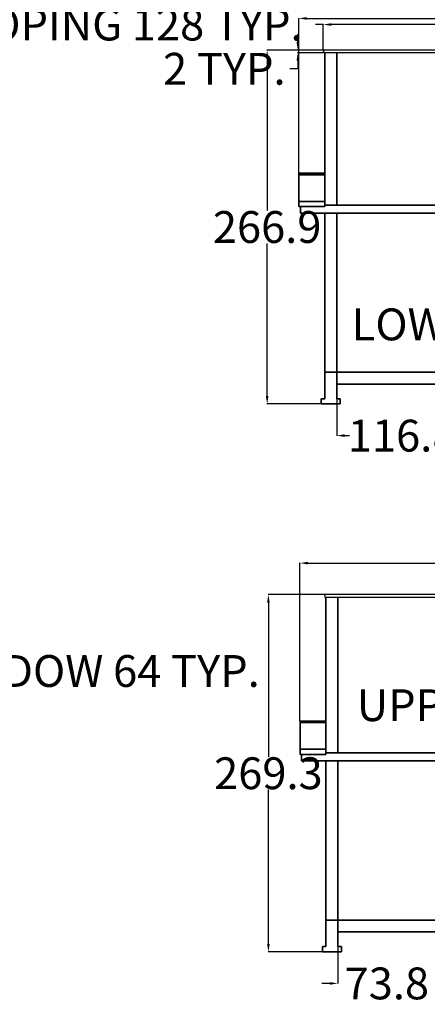
# Model space of a CAD drawing. Units: inches. Extents: x -15 to 1815, y 1023 to 2303.
# Tile 5 of 8: x 910 to 1217, y 1030 to 1773. Entities that reach past the tile are written whole.
import ezdxf

# ---------------------------------------------------------------- set-up
doc = ezdxf.new("R2010")
doc.units = ezdxf.units.IN
doc.header["$MEASUREMENT"] = 0
for name, color, linetype, lineweight in [('A-ANNO-DIMS', 2, 'Continuous', 18), ('A-FLOR', 7, 'Continuous', 35), ('A-ROOF', 7, 'Continuous', 25), ('A-SECT', 7, 'Continuous', 35), ('S-FNDN', 7, 'Continuous', 35)]:
    doc.layers.add(name, color=color, linetype=linetype, lineweight=lineweight)
doc.styles.get("Standard").update_dxf_attribs({"font": 'arial.ttf'})
doc.dimstyles.get("Standard").update_dxf_attribs({"dimtxt": 24, "dimasz": 6, "dimexe": 0.18, "dimexo": 0.0625, "dimgap": 0.09, "dimtad": 0, "dimtih": 1, "dimtoh": 1, "dimdec": 0, "dimzin": 0, "dimdsep": 46, "dimlunit": 3, "dimtxsty": 'Standard', "dimcen": 0.09, "dimadec": 0, "dimazin": 0, "dimtfac": 1, "dimtdec": 0, "dimtofl": 0, "dimtmove": 0, "dimatfit": 3, "dimfxl": 1, "dimtolj": 1, "dimtzin": 0, "dimarcsym": 0})

# ---------------------------------------------------------------- blocks, each defined once
blk = doc.blocks.new('COPING-ROUND-END')
for p, q in [((1.07, 2.13), (126.89, 2.13)), ((1.07, 0), (126.89, 0))]:
    blk.add_line(p, q)
for centre, start, end in [((1.07, 1.07), 90, 270), ((126.89, 1.07), 270, 90)]:
    blk.add_arc(centre, 1.07, start, end)
blk = doc.blocks.new('FOOTING-STRIP-SECTION')
for p, q in [((0, 0), (0, 3.98)), ((0, 3.98), (2.61, 3.98)), ((14.22, 0), (0, 0)), ((14.22, 3.98), (11.61, 3.98)), ((14.22, 0), (14.22, 3.98))]:
    blk.add_line(p, q)
blk = doc.blocks.new('*D41')
at = {"layer": 'A-ANNO-DIMS', "color": 0, "lineweight": -2, "transparency": 16777216}
for p, q in [((637.91, 1272.2), (637.91, 1281.94)), ((643.91, 1281.76), (696.08, 1281.76)), ((702.08, 1272.2), (702.08, 1281.94)), ((702.08, 1281.76), (708.08, 1281.76))]:
    blk.add_line(p, q, dxfattribs=at)
at = {"layer": 'A-ANNO-DIMS', "color": 0, "transparency": 16777216}
for points in [[(643.91, 1282.76), (643.91, 1280.76), (637.91, 1281.76)], [(696.08, 1282.76), (696.08, 1280.76), (702.08, 1281.76)]]:
    blk.add_solid(points, dxfattribs=at)
at = {"layer": 'Defpoints', "color": 0, "transparency": 16777216}
for p in [(702.08, 1281.76), (637.91, 1272.13), (702.08, 1272.13)]:
    blk.add_point(p, dxfattribs=at)
at = {"layer": 'A-ANNO-DIMS', "color": 0, "transparency": 16777216, "insert": (906.58, 1281.76), "char_height": 24, "attachment_point": 5}
blk.add_mtext('\\A1;UPPER WINDOW 64 TYP.', dxfattribs=at)
blk = doc.blocks.new('*D45')
at = {"layer": 'A-ANNO-DIMS', "color": 0, "lineweight": -2, "transparency": 16777216}
for p, q in [((1138.43, 1769.16), (1132.43, 1769.16)), ((1138.43, 1750.02), (1138.43, 1769.34)), ((1260.44, 1769.16), (1144.43, 1769.16)), ((1266.44, 1750.02), (1266.44, 1769.34))]:
    blk.add_line(p, q, dxfattribs=at)
at = {"layer": 'A-ANNO-DIMS', "color": 0, "transparency": 16777216}
for points in [[(1144.43, 1770.16), (1144.43, 1768.16), (1138.43, 1769.16)], [(1260.44, 1770.16), (1260.44, 1768.16), (1266.44, 1769.16)]]:
    blk.add_solid(points, dxfattribs=at)
at = {"layer": 'Defpoints', "color": 0, "transparency": 16777216}
for p in [(1138.43, 1769.16), (1138.43, 1749.96), (1266.44, 1749.96)]:
    blk.add_point(p, dxfattribs=at)
at = {"layer": 'A-ANNO-DIMS', "color": 0, "transparency": 16777216, "insert": (993.96, 1769.16), "char_height": 24, "attachment_point": 5}
blk.add_mtext('\\A1;COPING 128 TYP.', dxfattribs=at)
blk = doc.blocks.new('*D46')
at = {"layer": 'A-ANNO-DIMS', "color": 0, "lineweight": -2, "transparency": 16777216}
for p, q in [((1119.23, 1755.96), (1119.23, 1761.96)), ((1138.37, 1749.96), (1119.05, 1749.96)), ((1138.37, 1747.83), (1119.05, 1747.83)), ((1119.23, 1741.83), (1119.23, 1735.83)), ((1119.23, 1735.83), (1113.23, 1735.83))]:
    blk.add_line(p, q, dxfattribs=at)
at = {"layer": 'A-ANNO-DIMS', "color": 0, "transparency": 16777216}
for points in [[(1118.23, 1755.96), (1120.23, 1755.96), (1119.23, 1749.96)], [(1118.23, 1741.83), (1120.23, 1741.83), (1119.23, 1747.83)]]:
    blk.add_solid(points, dxfattribs=at)
at = {"layer": 'Defpoints', "color": 0, "transparency": 16777216}
for p in [(1119.23, 1747.83), (1138.43, 1749.96), (1138.43, 1747.83)]:
    blk.add_point(p, dxfattribs=at)
at = {"layer": 'A-ANNO-DIMS', "color": 0, "transparency": 16777216, "insert": (1063.85, 1735.83), "char_height": 24, "attachment_point": 5}
blk.add_mtext('\\A1;2 TYP.', dxfattribs=at)
blk = doc.blocks.new('*D49')
at = {"layer": 'A-ANNO-DIMS', "color": 0, "lineweight": -2, "transparency": 16777216}
for p, q in [((1313.13, 1579.08), (1324.05, 1579.08)), ((1323.87, 1573.08), (1323.87, 1555.58)), ((1323.87, 1513.08), (1323.87, 1530.57)), ((1313.13, 1507.08), (1324.05, 1507.08))]:
    blk.add_line(p, q, dxfattribs=at)
at = {"layer": 'A-ANNO-DIMS', "color": 0, "transparency": 16777216}
for points in [[(1322.87, 1573.08), (1324.87, 1573.08), (1323.87, 1579.08)], [(1322.87, 1513.08), (1324.87, 1513.08), (1323.87, 1507.08)]]:
    blk.add_solid(points, dxfattribs=at)
at = {"layer": 'Defpoints', "color": 0, "transparency": 16777216}
for p in [(1313.07, 1579.08), (1323.87, 1579.08), (1313.07, 1507.08)]:
    blk.add_point(p, dxfattribs=at)
at = {"layer": 'A-ANNO-DIMS', "color": 0, "transparency": 16777216, "insert": (1323.87, 1543.08), "char_height": 24, "attachment_point": 5}
blk.add_mtext('\\A1;LOWER DOOR 72 TYP.', dxfattribs=at)
blk = doc.blocks.new('*D51')
at = {"layer": 'A-ANNO-DIMS', "color": 0, "lineweight": -2, "transparency": 16777216}
for p, q in [((1314.04, 1291.99), (1324.95, 1291.99)), ((1324.77, 1285.99), (1324.77, 1268.5)), ((1324.77, 1225.99), (1324.77, 1243.49)), ((1314.04, 1219.99), (1324.95, 1219.99))]:
    blk.add_line(p, q, dxfattribs=at)
at = {"layer": 'A-ANNO-DIMS', "color": 0, "transparency": 16777216}
for points in [[(1323.77, 1285.99), (1325.77, 1285.99), (1324.77, 1291.99)], [(1323.77, 1225.99), (1325.77, 1225.99), (1324.77, 1219.99)]]:
    blk.add_solid(points, dxfattribs=at)
at = {"layer": 'Defpoints', "color": 0, "transparency": 16777216}
for p in [(1313.97, 1291.99), (1324.77, 1291.99), (1313.97, 1219.99)]:
    blk.add_point(p, dxfattribs=at)
at = {"layer": 'A-ANNO-DIMS', "color": 0, "transparency": 16777216, "insert": (1324.77, 1255.99), "char_height": 24, "attachment_point": 5}
blk.add_mtext('\\A1;UPPER DOOR 72 TYP.', dxfattribs=at)
blk = doc.blocks.new('*D103')
at = {"layer": 'A-ANNO-DIMS', "color": 0, "lineweight": -2, "transparency": 16777216}
for p, q in [((1119.96, 1657.14), (1119.96, 1773.99)), ((1125.96, 1773.81), (1297.05, 1773.81)), ((1550.46, 1773.81), (1379.37, 1773.81)), ((1556.46, 1657.14), (1556.46, 1773.99))]:
    blk.add_line(p, q, dxfattribs=at)
at = {"layer": 'A-ANNO-DIMS', "color": 0, "transparency": 16777216}
for points in [[(1125.96, 1774.81), (1125.96, 1772.81), (1119.96, 1773.81)], [(1550.46, 1774.81), (1550.46, 1772.81), (1556.46, 1773.81)]]:
    blk.add_solid(points, dxfattribs=at)
at = {"layer": 'Defpoints', "color": 0, "transparency": 16777216}
for p in [(1556.46, 1773.81), (1119.96, 1657.08), (1556.46, 1657.08)]:
    blk.add_point(p, dxfattribs=at)
at = {"layer": 'A-ANNO-DIMS', "color": 0, "transparency": 16777216, "insert": (1338.21, 1773.81), "char_height": 24, "attachment_point": 5}
blk.add_mtext('\\A1;436.5', dxfattribs=at)
blk = doc.blocks.new('*D104')
at = {"layer": 'A-ANNO-DIMS', "color": 0, "lineweight": -2, "transparency": 16777216}
for p, q in [((1139.44, 1749.96), (1095.93, 1749.96)), ((1096.11, 1743.96), (1096.11, 1628.86)), ((1096.11, 1489.08), (1096.11, 1604.17)), ((1136.83, 1483.08), (1095.93, 1483.08))]:
    blk.add_line(p, q, dxfattribs=at)
at = {"layer": 'A-ANNO-DIMS', "color": 0, "transparency": 16777216}
for points in [[(1095.11, 1743.96), (1097.11, 1743.96), (1096.11, 1749.96)], [(1095.11, 1489.08), (1097.11, 1489.08), (1096.11, 1483.08)]]:
    blk.add_solid(points, dxfattribs=at)
at = {"layer": 'Defpoints', "color": 0, "transparency": 16777216}
for p in [(1096.11, 1749.96), (1139.5, 1749.96), (1136.89, 1483.08)]:
    blk.add_point(p, dxfattribs=at)
at = {"layer": 'A-ANNO-DIMS', "color": 0, "transparency": 16777216, "insert": (1096.11, 1616.52), "char_height": 24, "attachment_point": 5}
blk.add_mtext('\\A1;266.9', dxfattribs=at)
blk = doc.blocks.new('*D107')
at = {"layer": 'A-ANNO-DIMS', "color": 0, "lineweight": -2, "transparency": 16777216}
for p, q in [((1148.5, 1507.01), (1148.5, 1459.05)), ((1265.32, 1507.01), (1265.32, 1459.05)), ((1154.5, 1459.23), (1158.26, 1459.23)), ((1259.32, 1459.23), (1255.57, 1459.23))]:
    blk.add_line(p, q, dxfattribs=at)
at = {"layer": 'A-ANNO-DIMS', "color": 0, "transparency": 16777216}
for points in [[(1154.5, 1460.23), (1154.5, 1458.23), (1148.5, 1459.23)], [(1259.32, 1460.23), (1259.32, 1458.23), (1265.32, 1459.23)]]:
    blk.add_solid(points, dxfattribs=at)
at = {"layer": 'Defpoints', "color": 0, "transparency": 16777216}
for p in [(1148.5, 1507.08), (1265.32, 1507.08), (1265.32, 1459.23)]:
    blk.add_point(p, dxfattribs=at)
at = {"layer": 'A-ANNO-DIMS', "color": 0, "transparency": 16777216, "insert": (1206.91, 1459.23), "char_height": 24, "attachment_point": 5}
blk.add_mtext('\\A1;116.82', dxfattribs=at)
blk = doc.blocks.new('*D113')
at = {"layer": 'A-ANNO-DIMS', "color": 0, "lineweight": -2, "transparency": 16777216}
for p, q in [((1120.86, 1244.06), (1120.86, 1363.3)), ((1126.86, 1363.12), (1297.96, 1363.12)), ((1551.37, 1363.12), (1380.27, 1363.12)), ((1557.37, 1244.06), (1557.37, 1363.3))]:
    blk.add_line(p, q, dxfattribs=at)
at = {"layer": 'A-ANNO-DIMS', "color": 0, "transparency": 16777216}
for points in [[(1126.86, 1364.12), (1126.86, 1362.12), (1120.86, 1363.12)], [(1551.37, 1364.12), (1551.37, 1362.12), (1557.37, 1363.12)]]:
    blk.add_solid(points, dxfattribs=at)
at = {"layer": 'Defpoints', "color": 0, "transparency": 16777216}
for p in [(1557.37, 1363.12), (1120.86, 1243.99), (1557.37, 1243.99)]:
    blk.add_point(p, dxfattribs=at)
at = {"layer": 'A-ANNO-DIMS', "color": 0, "transparency": 16777216, "insert": (1339.12, 1363.12), "char_height": 24, "attachment_point": 5}
blk.add_mtext('\\A1;436.5', dxfattribs=at)
blk = doc.blocks.new('*D114')
at = {"layer": 'A-ANNO-DIMS', "color": 0, "lineweight": -2, "transparency": 16777216}
for p, q in [((1140.35, 1339.32), (1096.88, 1339.32)), ((1097.06, 1333.32), (1097.06, 1217.01)), ((1097.06, 1075.99), (1097.06, 1192.31)), ((1137.74, 1069.99), (1096.88, 1069.99))]:
    blk.add_line(p, q, dxfattribs=at)
at = {"layer": 'A-ANNO-DIMS', "color": 0, "transparency": 16777216}
for points in [[(1096.06, 1333.32), (1098.06, 1333.32), (1097.06, 1339.32)], [(1096.06, 1075.99), (1098.06, 1075.99), (1097.06, 1069.99)]]:
    blk.add_solid(points, dxfattribs=at)
at = {"layer": 'Defpoints', "color": 0, "transparency": 16777216}
for p in [(1097.06, 1339.32), (1140.41, 1339.32), (1137.8, 1069.99)]:
    blk.add_point(p, dxfattribs=at)
at = {"layer": 'A-ANNO-DIMS', "color": 0, "transparency": 16777216, "insert": (1097.06, 1204.66), "char_height": 24, "attachment_point": 5}
blk.add_mtext('\\A1;269.3', dxfattribs=at)
blk = doc.blocks.new('*D119')
at = {"layer": 'A-ANNO-DIMS', "color": 0, "lineweight": -2, "transparency": 16777216}
for p, q in [((1223.21, 1178.86), (1223.21, 1046.01)), ((1149.41, 1093.93), (1149.41, 1046.01)), ((1143.41, 1046.19), (1137.41, 1046.19)), ((1229.21, 1046.19), (1235.21, 1046.19))]:
    blk.add_line(p, q, dxfattribs=at)
at = {"layer": 'A-ANNO-DIMS', "color": 0, "transparency": 16777216}
for points in [[(1143.41, 1047.19), (1143.41, 1045.19), (1149.41, 1046.19)], [(1229.21, 1047.19), (1229.21, 1045.19), (1223.21, 1046.19)]]:
    blk.add_solid(points, dxfattribs=at)
at = {"layer": 'Defpoints', "color": 0, "transparency": 16777216}
for p in [(1223.21, 1178.93), (1149.41, 1093.99), (1223.21, 1046.19)]:
    blk.add_point(p, dxfattribs=at)
at = {"layer": 'A-ANNO-DIMS', "color": 0, "transparency": 16777216, "insert": (1186.31, 1046.19), "char_height": 24, "attachment_point": 5}
blk.add_mtext('\\A1;73.8', dxfattribs=at)

msp = doc.modelspace()

# ---------------------------------------------------------------- linework, layer by layer
at = {"layer": 'A-FLOR'}
for p, q in [((1139.4997, 1657.0773), (1119.956, 1657.0773)), ((1119.956, 1657.0773), (1119.956, 1631.8931)), ((1139.4997, 1657.0773), (1119.956, 1657.0773)), ((1139.4997, 1655.9681), (1119.956, 1655.9681)), ((1139.4997, 1635.8405), (1119.956, 1635.8405)), ((1139.4997, 1631.8931), (1119.956, 1631.8931)), ((1121.1268, 1631.8931), (1121.1268, 1627.0773)), ((1139.4997, 1627.0773), (1121.1268, 1627.0773)), ((1265.3241, 1633.0773), (1139.4997, 1633.0773)), ((1265.3241, 1627.0773), (1139.4997, 1627.0773)), ((1265.3241, 1507.0773), (1139.4997, 1507.0773)), ((1148.4997, 1507.0773), (1139.4997, 1507.0773)), ((1265.3241, 1498.0773), (1148.4997, 1498.0773)), ((1140.4077, 1243.9947), (1120.864, 1243.9947)), ((1120.864, 1243.9947), (1120.864, 1218.8104)), ((1140.4077, 1243.9947), (1120.864, 1243.9947)), ((1140.4077, 1242.8854), (1120.864, 1242.8854)), ((1140.4077, 1222.7579), (1120.864, 1222.7579)), ((1140.4077, 1218.8104), (1120.864, 1218.8104)), ((1122.0348, 1218.8104), (1122.0348, 1213.9947)), ((1266.2321, 1219.9947), (1140.4077, 1219.9947)), ((1140.4077, 1213.9947), (1122.0348, 1213.9947)), ((1266.2321, 1213.9947), (1140.4077, 1213.9947)), ((1266.2321, 1093.9947), (1140.4077, 1093.9947)), ((1266.2321, 1084.9947), (1149.4077, 1084.9947))]:
    msp.add_line(p, q, dxfattribs=at)
at = {"layer": 'A-SECT'}
for p, q in [((1139.4997, 1747.8268), (1139.4997, 1631.8931)), ((1148.4997, 1747.8268), (1148.4997, 1633.0773)), ((1139.4997, 1627.0773), (1139.4997, 1507.0773)), ((1148.4997, 1627.0773), (1148.4997, 1507.0773)), ((1139.4997, 1582.655), (1139.4997, 1487.0609)), ((1148.4997, 1582.655), (1148.4997, 1487.0609)), ((1140.4077, 1337.1888), (1140.4077, 1218.8104)), ((1149.4077, 1337.1888), (1149.4077, 1219.9947)), ((1140.4077, 1213.9947), (1140.4077, 1093.9947)), ((1149.4077, 1213.9947), (1149.4077, 1093.9947)), ((1140.4077, 1169.5723), (1140.4077, 1093.9947)), ((1149.4077, 1169.5723), (1149.4077, 1093.9947))]:
    msp.add_line(p, q, dxfattribs=at)
at = {"layer": 'S-FNDN'}
for p, q in [((1139.4997, 1582.655), (1139.4997, 1487.0609)), ((1140.4077, 1169.5723), (1140.4077, 1073.9782)), ((1140.4077, 1169.5723), (1140.4077, 1073.9782)), ((1149.4077, 1169.5723), (1149.4077, 1073.9782))]:
    msp.add_line(p, q, dxfattribs=at)

# ---------------------------------------------------------------- block references
at = {"layer": 'A-ROOF', "rotation": 180}
for p in [(1266.39, 1749.9585), (1267.298, 1339.3206)]:
    msp.add_blockref('COPING-ROUND-END', p, dxfattribs=at)
at = {"layer": 'S-FNDN'}
for p in [(1136.8895, 1483.0773), (1137.7975, 1069.9947)]:
    msp.add_blockref('FOOTING-STRIP-SECTION', p, dxfattribs=at)

# ---------------------------------------------------------------- dimensions: what is measured, and where the dimension line sits
at = {"layer": 'A-ANNO-DIMS'}
for base, p1, p2, angle, text, picture, middle in [((1138.4338, 1769.1591), (1266.4376, 1749.9585), (1138.4338, 1749.9585), 180, 'COPING <> TYP.', '*D45', (993.9591, 1769.1591)), ((1119.2332, 1747.8268), (1138.4338, 1749.9585), (1138.4338, 1747.8268), 270, '<> TYP.', '*D46', (1063.8499, 1735.8268)), ((1323.8659, 1579.0773), (1313.0659, 1507.0773), (1313.0659, 1579.0773), 90, 'LOWER DOOR <> TYP.', '*D49', (1323.8659, 1543.0773)), ((1324.7739, 1291.9947), (1313.9739, 1219.9947), (1313.9739, 1291.9947), 90, 'UPPER DOOR <> TYP.', '*D51', (1324.7739, 1255.9947))]:
    dim = msp.add_linear_dim(base=base, p1=p1, p2=p2, angle=angle, text=text, dimstyle='Standard', override={"dimdec": 0, "dimlfac": 1, "dimrnd": 0, "dimzin": 0, "dimdsep": 46, "dimlunit": 2}, dxfattribs=at)
    dim.commit()
    dim.dimension.update_dxf_attribs({"geometry": picture, "text_midpoint": middle})
for base, p1, p2, override, picture, middle in [((1556.4613, 1773.8085), (1119.956, 1657.0773), (1556.4613, 1657.0773), {"dimdec": 1, "dimlfac": 1, "dimrnd": 0, "dimzin": 0, "dimdsep": 46, "dimlunit": 2}, '*D103', (1338.2086, 1773.8085)), ((1265.3241, 1459.2273), (1148.4997, 1507.0773), (1265.3241, 1507.0773), {"dimdec": 2, "dimlfac": 1, "dimrnd": 0, "dimzin": 0, "dimdsep": 46, "dimlunit": 2}, '*D107', (1206.9119, 1459.2273)), ((1557.3693, 1363.1206), (1120.864, 1243.9947), (1557.3693, 1243.9947), {"dimdec": 1, "dimlfac": 1, "dimrnd": 0, "dimzin": 0, "dimdsep": 46, "dimlunit": 2}, '*D113', (1339.1166, 1363.1206)), ((1223.2102, 1046.1947), (1149.4077, 1093.9947), (1223.2102, 1178.9271), {"dimdec": 1, "dimlfac": 1, "dimrnd": 0, "dimzin": 0, "dimdsep": 46, "dimlunit": 2}, '*D119', (1186.309, 1046.1947))]:
    dim = msp.add_linear_dim(base=base, p1=p1, p2=p2, dimstyle='Standard', override=override, dxfattribs=at)
    dim.commit()
    dim.dimension.update_dxf_attribs({"geometry": picture, "text_midpoint": middle})
for base, p1, p2, picture, middle in [((1096.106, 1749.9585), (1136.8895, 1483.0773), (1139.4997, 1749.9585), '*D104', (1096.106, 1616.5179)), ((1097.064, 1339.3206), (1137.7975, 1069.9947), (1140.4077, 1339.3206), '*D114', (1097.064, 1204.6576))]:
    dim = msp.add_linear_dim(base=base, p1=p1, p2=p2, angle=90, dimstyle='Standard', override={"dimdec": 1, "dimlfac": 1, "dimrnd": 0, "dimzin": 0, "dimdsep": 46, "dimlunit": 2}, dxfattribs=at)
    dim.commit()
    dim.dimension.update_dxf_attribs({"geometry": picture, "text_midpoint": middle})
dim = msp.add_linear_dim(base=(702.0758, 1281.7576), p1=(637.9105, 1272.1328), p2=(702.0758, 1272.1328), text='UPPER WINDOW <> TYP.', dimstyle='Standard', override={"dimdec": 0, "dimlfac": 1, "dimrnd": 0, "dimzin": 0, "dimdsep": 46, "dimlunit": 2}, dxfattribs=at)
dim.commit()
dim.dimension.update_dxf_attribs({"geometry": '*D41', "text_midpoint": (906.5833, 1281.7576)})

doc.saveas('drawing.dxf')
